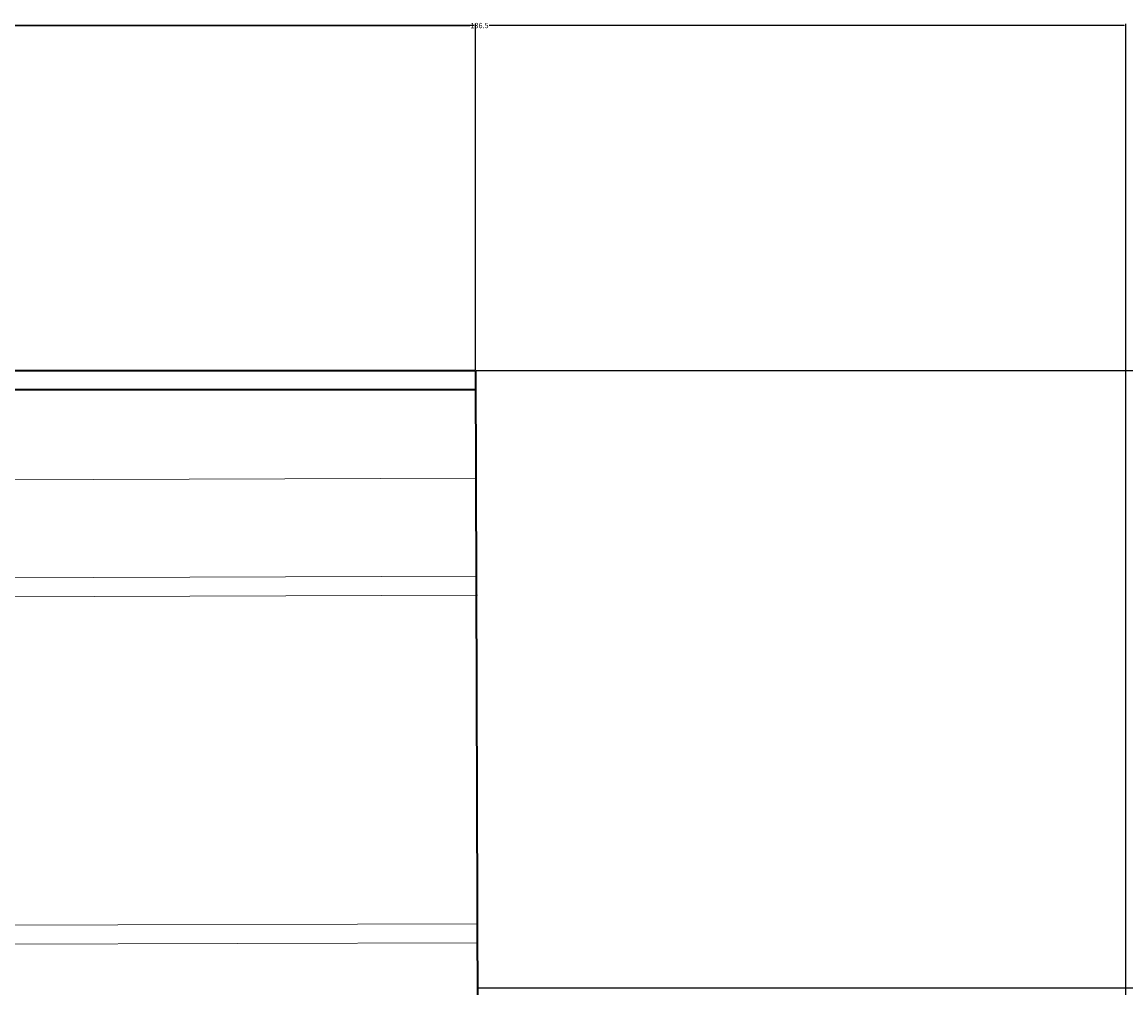
# Model space of a CAD drawing. Units: inches. Extents: x -26 to 776, y -22 to 650.
# Tile 40 of 62: x 309 to 426, y 548 to 650. Entities that reach past the tile are written whole.
import ezdxf

# ---------------------------------------------------------------- set-up
doc = ezdxf.new("R2010")
doc.units = ezdxf.units.IN
doc.header["$MEASUREMENT"] = 0
for name, color, linetype, lineweight in [('A-ANNO-DIMS', 2, 'Continuous', 18), ('A-ROOF', 7, 'Continuous', 35), ('A-WALL', 7, 'Continuous', 35), ('A-WALL-TRIM', 7, 'Continuous', 18)]:
    doc.layers.add(name, color=color, linetype=linetype, lineweight=lineweight)
doc.styles.get("Standard").update_dxf_attribs({"font": 'arial.ttf'})
doc.dimstyles.get("Standard").update_dxf_attribs({"dimtxt": 0.5625, "dimasz": 0.18, "dimexe": 0.18, "dimexo": 0.0625, "dimgap": 0.09, "dimtad": 0, "dimtih": 1, "dimtoh": 1, "dimdec": 4, "dimzin": 0, "dimdsep": 46, "dimlunit": 4, "dimtxsty": 'Standard', "dimcen": 0.09, "dimadec": 0, "dimazin": 0, "dimtfac": 1, "dimtdec": 4, "dimtofl": 0, "dimtmove": 0, "dimatfit": 3, "dimfxl": 1, "dimtolj": 1, "dimtzin": 0, "dimarcsym": 0})

# ---------------------------------------------------------------- blocks, each defined once
blk = doc.blocks.new('*D18')
at = {"layer": 'A-ANNO-DIMS', "color": 0, "lineweight": -2, "transparency": 16777216}
for p, q in [((191.68, 613.33), (191.68, 649.86)), ((191.86, 649.68), (273.36, 649.68)), ((356.89, 649.68), (275.38, 649.68)), ((357.07, 613.33), (357.07, 649.86))]:
    blk.add_line(p, q, dxfattribs=at)
at = {"layer": 'A-ANNO-DIMS', "color": 0, "transparency": 16777216}
for points in [[(191.86, 649.71), (191.86, 649.65), (191.68, 649.68)], [(356.89, 649.71), (356.89, 649.65), (357.07, 649.68)]]:
    blk.add_solid(points, dxfattribs=at)
at = {"layer": 'Defpoints', "color": 0, "transparency": 16777216}
for p in [(357.07, 649.68), (191.68, 613.27), (357.07, 613.27)]:
    blk.add_point(p, dxfattribs=at)
at = {"layer": 'A-ANNO-DIMS', "color": 0, "transparency": 16777216, "insert": (274.37, 649.68), "char_height": 0.562, "attachment_point": 5}
blk.add_mtext('\\A1;165.4', dxfattribs=at)
blk = doc.blocks.new('*D32')
at = {"layer": 'A-ANNO-DIMS', "color": 0, "lineweight": -2, "transparency": 16777216}
for p, q in [((357.13, 613.27), (775.34, 613.27)), ((775.16, 613.09), (775.16, 581.06)), ((775.16, 548.28), (775.16, 580.31)), ((357.37, 548.1), (775.34, 548.1))]:
    blk.add_line(p, q, dxfattribs=at)
at = {"layer": 'A-ANNO-DIMS', "color": 0, "transparency": 16777216}
for points in [[(775.13, 613.09), (775.19, 613.09), (775.16, 613.27)], [(775.13, 548.28), (775.19, 548.28), (775.16, 548.1)]]:
    blk.add_solid(points, dxfattribs=at)
at = {"layer": 'Defpoints', "color": 0, "transparency": 16777216}
for p in [(357.07, 613.27), (775.16, 613.27), (357.3, 548.1)]:
    blk.add_point(p, dxfattribs=at)
at = {"layer": 'A-ANNO-DIMS', "color": 0, "transparency": 16777216, "insert": (775.16, 580.69), "char_height": 0.562, "attachment_point": 5}
blk.add_mtext('\\A1;65.17', dxfattribs=at)
blk = doc.blocks.new('*D33')
at = {"layer": 'A-ANNO-DIMS', "color": 0, "lineweight": -2, "transparency": 16777216}
for p, q in [((357.37, 548.1), (775.34, 548.1)), ((775.16, 547.92), (775.16, 538.64)), ((775.16, 528.6), (775.16, 537.88)), ((357.37, 528.42), (775.34, 528.42))]:
    blk.add_line(p, q, dxfattribs=at)
at = {"layer": 'A-ANNO-DIMS', "color": 0, "transparency": 16777216}
for points in [[(775.13, 547.92), (775.19, 547.92), (775.16, 548.1)], [(775.13, 528.6), (775.19, 528.6), (775.16, 528.42)]]:
    blk.add_solid(points, dxfattribs=at)
at = {"layer": 'Defpoints', "color": 0, "transparency": 16777216}
for p in [(357.3, 548.1), (775.16, 548.1), (357.3, 528.42)]:
    blk.add_point(p, dxfattribs=at)
at = {"layer": 'A-ANNO-DIMS', "color": 0, "transparency": 16777216, "insert": (775.16, 538.26), "char_height": 0.562, "attachment_point": 5}
blk.add_mtext('\\A1;19.676', dxfattribs=at)
blk = doc.blocks.new('*D39')
at = {"layer": 'A-ANNO-DIMS', "color": 0, "lineweight": -2, "transparency": 16777216}
for p, q in [((289.24, 15.54), (289.24, 649.86)), ((289.42, 649.68), (356.48, 649.68)), ((425.56, 649.68), (358.51, 649.68)), ((425.74, 15.54), (425.74, 649.86))]:
    blk.add_line(p, q, dxfattribs=at)
at = {"layer": 'A-ANNO-DIMS', "color": 0, "transparency": 16777216}
for points in [[(289.42, 649.71), (289.42, 649.65), (289.24, 649.68)], [(425.56, 649.71), (425.56, 649.65), (425.74, 649.68)]]:
    blk.add_solid(points, dxfattribs=at)
at = {"layer": 'Defpoints', "color": 0, "transparency": 16777216}
for p in [(425.74, 649.68), (289.24, 15.48), (425.74, 15.48)]:
    blk.add_point(p, dxfattribs=at)
at = {"layer": 'A-ANNO-DIMS', "color": 0, "transparency": 16777216, "insert": (357.49, 649.68), "char_height": 0.562, "attachment_point": 5}
blk.add_mtext('\\A1;136.5', dxfattribs=at)

msp = doc.modelspace()

# ---------------------------------------------------------------- linework, layer by layer
at = {"layer": 'A-ROOF'}
for p, q in [((191.6782, 613.2713), (357.0669, 613.2713)), ((191.6782, 611.2713), (357.0669, 611.2713))]:
    msp.add_line(p, q, dxfattribs=at)
at = {"layer": 'A-WALL'}
msp.add_line((357.0669, 613.2713), (357.4929, 478.1838), dxfattribs=at)
at = {"layer": 'A-WALL-TRIM'}
for p, q in [((191.8658, 601.3674), (357.1028, 601.8885)), ((191.6719, 591.0323), (357.2511, 591.5545)), ((191.6782, 589.0323), (357.2574, 589.5545)), ((191.6719, 554.3491), (357.2511, 554.8713)), ((191.6782, 552.3491), (357.2574, 552.8713))]:
    msp.add_line(p, q, dxfattribs=at)

# ---------------------------------------------------------------- dimensions: what is measured, and where the dimension line sits
at = {"layer": 'A-ANNO-DIMS'}
for base, p1, p2, picture, middle in [((357.0669, 649.6763), (191.6782, 613.2713), (357.0669, 613.2713), '*D18', (274.3725, 649.6763)), ((425.7434, 649.6763), (289.2424, 15.4824), (425.7434, 15.4824), '*D39', (357.4929, 649.6763))]:
    dim = msp.add_linear_dim(base=base, p1=p1, p2=p2, dimstyle='Standard', override={"dimdec": 1, "dimlfac": 1, "dimrnd": 0, "dimzin": 0, "dimdsep": 46, "dimlunit": 2}, dxfattribs=at)
    dim.commit()
    dim.dimension.update_dxf_attribs({"geometry": picture, "text_midpoint": middle})
for base, p1, p2, override, picture, middle in [((775.1553, 613.2713), (357.3034, 548.0996), (357.0669, 613.2713), {"dimdec": 2, "dimlfac": 1, "dimrnd": 0, "dimzin": 0, "dimdsep": 46, "dimlunit": 2}, '*D32', (775.1553, 580.6855)), ((775.1553, 548.0996), (357.3034, 528.4233), (357.3034, 548.0996), {"dimdec": 3, "dimlfac": 1, "dimrnd": 0, "dimzin": 0, "dimdsep": 46, "dimlunit": 2}, '*D33', (775.1553, 538.2614))]:
    dim = msp.add_linear_dim(base=base, p1=p1, p2=p2, angle=90, dimstyle='Standard', override=override, dxfattribs=at)
    dim.commit()
    dim.dimension.update_dxf_attribs({"geometry": picture, "text_midpoint": middle})

doc.saveas('drawing.dxf')
